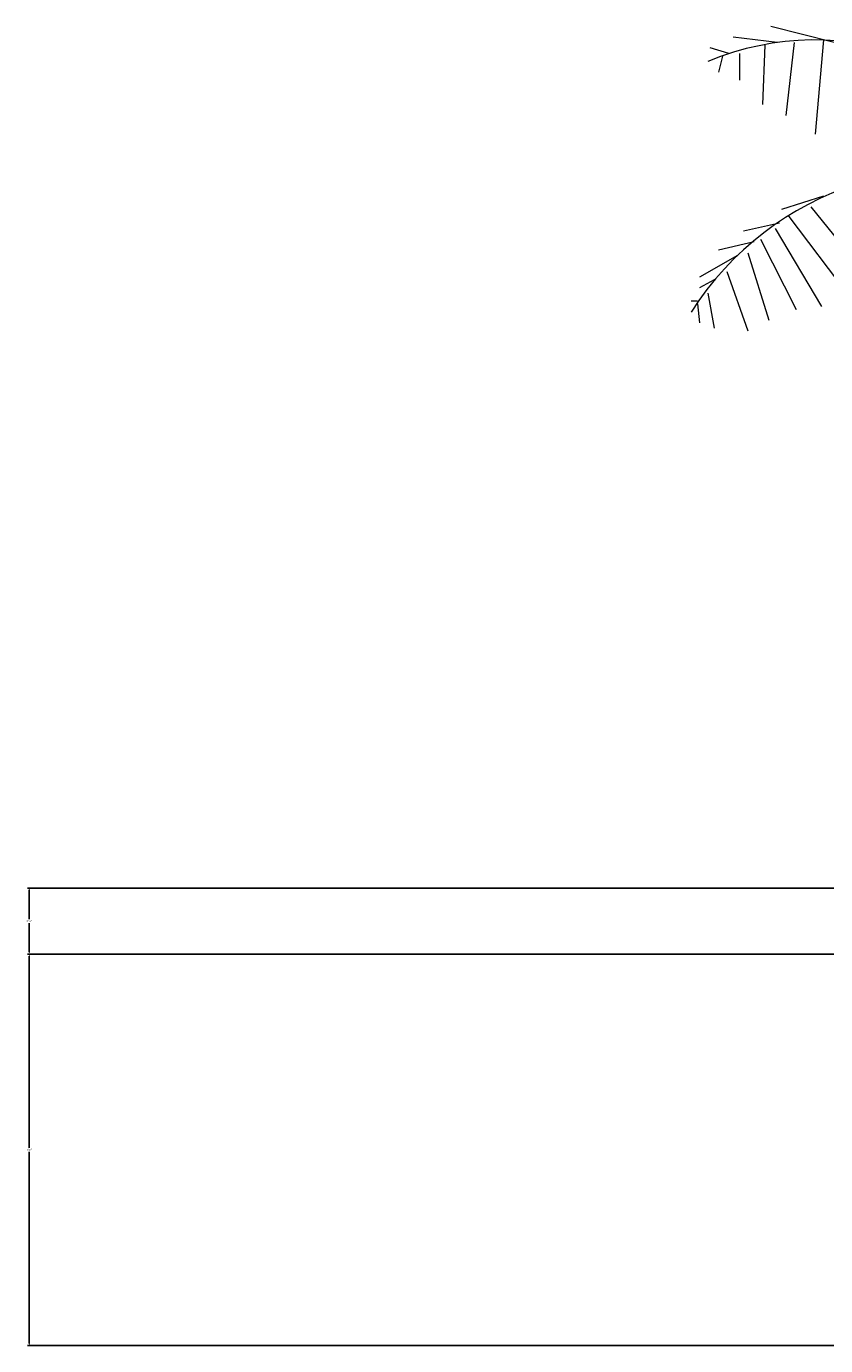
# Model space of a CAD drawing. Units: inches. Extents: x 37 to 824, y -700 to 234.
# Tile 2 of 77: x 37 to 110, y -532 to -410. Entities that reach past the tile are written whole.
import ezdxf

# ---------------------------------------------------------------- set-up
doc = ezdxf.new("R2010")
doc.units = ezdxf.units.IN
doc.header["$MEASUREMENT"] = 0
doc.layers.add('A-ANNO-DIMS', color=2, linetype='Continuous', lineweight=18)
doc.layers.add('A-SITE-PLNT', color=3, linetype='Continuous', lineweight=13)
doc.styles.get("Standard").update_dxf_attribs({"font": 'arial.ttf'})
doc.dimstyles.get("Standard").update_dxf_attribs({"dimtxt": 0.18, "dimasz": 0.18, "dimexe": 0.18, "dimexo": 0.0625, "dimgap": 0.09, "dimtad": 0, "dimtih": 1, "dimtoh": 1, "dimdec": 1, "dimzin": 0, "dimdsep": 46, "dimlunit": 4, "dimtxsty": 'Standard', "dimcen": 0.09, "dimadec": 0, "dimazin": 0, "dimtfac": 1, "dimtdec": 1, "dimtofl": 0, "dimtmove": 0, "dimatfit": 3, "dimfxl": 1, "dimtolj": 1, "dimtzin": 0, "dimarcsym": 0})

# ---------------------------------------------------------------- blocks, each defined once
blk = doc.blocks.new('*U34')
for p, q in [((-20.064, 191.751), (-25.863, 193.238)), ((-25.283, 191.751), (-29.342, 192.246)), ((-23.737, 191.751), (-24.51, 185.06)), ((-21.031, 191.998), (-21.804, 183.325)), ((-29.729, 190.759), (-31.469, 191.255)), ((-30.309, 190.512), (-30.695, 189.025)), ((-28.763, 190.759), (-28.763, 188.281)), ((-26.443, 191.503), (-26.636, 186.051)), ((-21.031, 177.626), (-24.897, 176.387)), ((-22.191, 176.635), (-16.391, 169.448)), ((-25.09, 175.148), (-28.376, 174.404)), ((-24.317, 175.891), (-18.711, 168.457)), ((-26.829, 173.661), (-23.544, 167.218)), ((-25.476, 174.652), (-21.224, 167.466)), ((-27.409, 173.413), (-30.695, 172.67)), ((-27.989, 172.422), (-26.056, 166.227)), ((-28.956, 172.174), (-32.435, 170.192)), ((-31.082, 169.944), (-32.435, 169.2)), ((-29.922, 170.687), (-27.989, 165.235)), ((-31.662, 168.705), (-31.082, 165.483)), ((-32.628, 167.961), (-33.208, 167.961)), ((-32.628, 167.713), (-32.435, 165.979))]:
    blk.add_line(p, q)
for centre, radius, start, end in [((-21.738, 166.094), 25.899, 27.67115, 112.5305), ((-9.259, 151.732), 28.386, 68.38311, 147.5322)]:
    blk.add_arc(centre, radius, start, end)
blk = doc.blocks.new('*D96')
at = {"layer": 'A-ANNO-DIMS', "color": 0, "lineweight": -2, "ltscale": 0.5, "transparency": 16777216}
for p, q in [((205.01, -489.63), (36.85, -489.63)), ((37.03, -489.81), (37.03, -492.49)), ((37.03, -495.53), (37.03, -492.85)), ((211.96, -495.71), (36.85, -495.71))]:
    blk.add_line(p, q, dxfattribs=at)
at = {"layer": 'A-ANNO-DIMS', "color": 0, "ltscale": 0.5, "transparency": 16777216}
for points in [[(37, -489.81), (37.06, -489.81), (37.03, -489.63)], [(37, -495.53), (37.06, -495.53), (37.03, -495.71)]]:
    blk.add_solid(points, dxfattribs=at)
at = {"layer": 'Defpoints', "color": 0, "ltscale": 0.5, "transparency": 16777216}
for p in [(205.08, -489.63), (37.03, -495.71), (212.03, -495.71)]:
    blk.add_point(p, dxfattribs=at)
at = {"layer": 'A-ANNO-DIMS', "color": 0, "ltscale": 0.5, "transparency": 16777216, "insert": (37.03, -492.67), "char_height": 0.18, "attachment_point": 5}
blk.add_mtext('\\A1;0\'-6"', dxfattribs=at)
blk = doc.blocks.new('*D97')
at = {"layer": 'A-ANNO-DIMS', "color": 0, "lineweight": -2, "ltscale": 0.5, "transparency": 16777216}
for p, q in [((211.96, -495.71), (36.85, -495.71)), ((37.03, -495.89), (37.03, -513.53)), ((37.03, -531.53), (37.03, -513.9)), ((211.96, -531.71), (36.85, -531.71))]:
    blk.add_line(p, q, dxfattribs=at)
at = {"layer": 'A-ANNO-DIMS', "color": 0, "ltscale": 0.5, "transparency": 16777216}
for points in [[(37, -495.89), (37.06, -495.89), (37.03, -495.71)], [(37, -531.53), (37.06, -531.53), (37.03, -531.71)]]:
    blk.add_solid(points, dxfattribs=at)
at = {"layer": 'Defpoints', "color": 0, "ltscale": 0.5, "transparency": 16777216}
for p in [(212.03, -495.71), (37.03, -531.71), (212.03, -531.71)]:
    blk.add_point(p, dxfattribs=at)
at = {"layer": 'A-ANNO-DIMS', "color": 0, "ltscale": 0.5, "transparency": 16777216, "insert": (37.03, -513.71), "char_height": 0.18, "attachment_point": 5}
blk.add_mtext('\\A1;3\'-0"', dxfattribs=at)

msp = doc.modelspace()

# ---------------------------------------------------------------- block references
at = {"layer": 'A-SITE-PLNT'}
msp.add_blockref('*U34', (131.08, -603.63), dxfattribs=at)

# ---------------------------------------------------------------- dimensions: what is measured, and where the dimension line sits
at = {"layer": 'A-ANNO-DIMS', "ltscale": 0.5}
for base, p1, p2, picture, middle in [((37.03, -495.71), (205.08, -489.63), (212.03, -495.71), '*D96', (37.03, -492.67)), ((37.03, -531.71), (212.03, -495.71), (212.03, -531.71), '*D97', (37.03, -513.71))]:
    dim = msp.add_linear_dim(base=base, p1=p1, p2=p2, angle=90, dimstyle='Standard', override={"dimdec": 1, "dimlfac": 1, "dimrnd": 0, "dimzin": 1, "dimdsep": 46, "dimlunit": 4, "dimfrac": 2}, dxfattribs=at)
    dim.commit()
    dim.dimension.update_dxf_attribs({"geometry": picture, "text_midpoint": middle})

doc.saveas('drawing.dxf')
